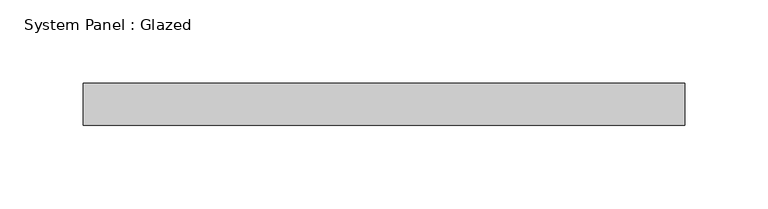
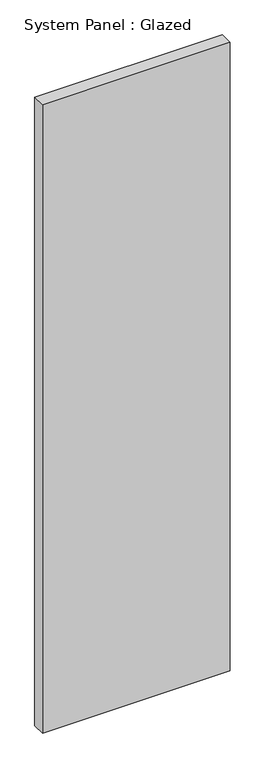
"""IFC4 building model written with IfcOpenShell, lengths in millimetres: plate geometry, System Panel : Glazed."""

from ifc_helpers import new_model, si_unit, origin, origin_with_axes, place, context, project, spatial, polyline, outline, extrude, source, transform, mapped, element, save


def system_panel_glazed_fc3a3408(model_context):
    return source(origin(), model_context, "Body", "SweptSolid", [
        extrude(outline(polyline([(180.975, 19.05), (-180.975, 19.05), (-180.975, 44.45), (180.975, 44.45), (180.975, 19.05)])), origin_with_axes(), (0.0, 0.0, 1.0), 1281.8373989),
    ])


if __name__ == "__main__":
    model = new_model("IFC4")
    model_context = context("Model", 3, world=origin())
    ifc_project = project(units=[si_unit("LENGTHUNIT", "METRE", prefix="MILLI")], contexts=[model_context])
    site = spatial("IfcSite", under=ifc_project)
    building = spatial("IfcBuilding", under=site)
    placement = place(None, origin())
    system_panel_glazed_shape = system_panel_glazed_fc3a3408(model_context)
    element("IfcPlate", 1, ObjectType="System Panel : Glazed", at=placement, inside=building, context=model_context, shape_type="MappedRepresentation", body=[
        mapped(system_panel_glazed_shape, transform((0.0, 0.0, 0.0), x_axis=(1.0, 0.0, 0.0), y_axis=(0.0, 1.0, 0.0), z_axis=(0.0, 0.0, 1.0))),
    ])
    save(model, "model.ifc")

# Revit data of these elements
# Type "System Panel : Glazed"
#   Construction Type Id = "GSP4R"
#   Analytic Construction = "1/8 in Pilkington single glazing"
#   Visual Light Transmittance = 0.9
#   Solar Heat Gain Coefficient = 0.86
#   Heat Transfer Coefficient (U) = 1.18115 BTU/(h·ft²·°F)
#   Define Thermal Properties by = 1
# Element 1 (IfcPlate, "System Panel : Glazed")
#   Materials on its faces: "Glass"
# Materials
#   "Glass": class "Glass", colour RGB 0 128 192, transparency 0.75, Description = "Soda Lime Glass", Cost = 0
